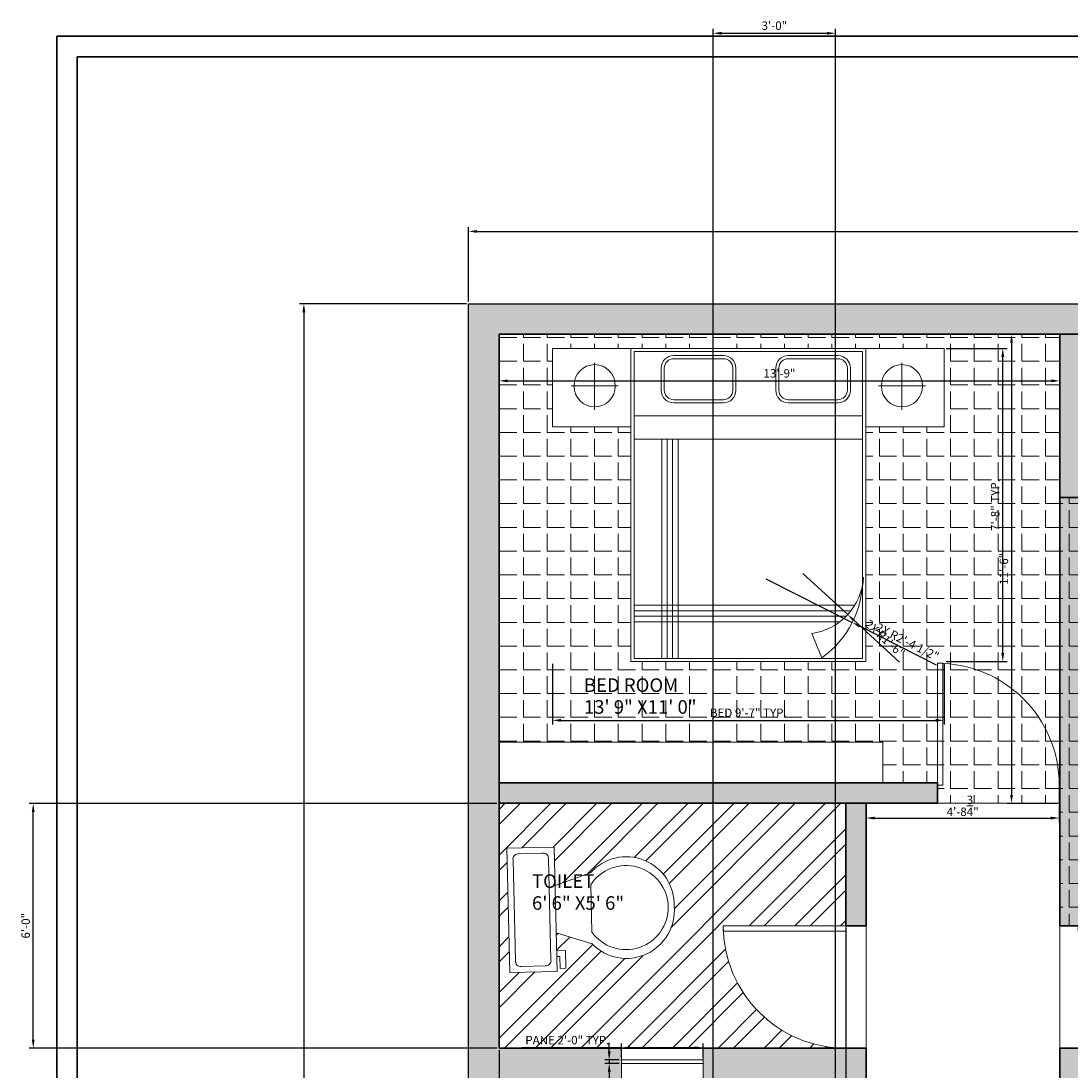
# Model space of a CAD drawing. Units: inches. Extents: x 2004 to 2661, y 1548 to 2351.
# Tile 4 of 5: x 2004 to 2312, y 2040 to 2349. Entities that reach past the tile are written whole.
import ezdxf

# ---------------------------------------------------------------- set-up
doc = ezdxf.new("R2010")
doc.units = ezdxf.units.IN
for name, color, linetype, lineweight in [('A-ANNO-DIMS', 2, 'Continuous', 18), ('A-ANNO-TTLB', 7, 'Continuous', 35), ('A-AREA-IDEN', 7, 'Continuous', 18), ('A-DOOR', 3, 'Continuous', 18), ('A-FLOR-CASE', 8, 'Continuous', 18), ('A-FLOR-FIXT', 9, 'Continuous', 18), ('A-FURN', 8, 'Continuous', 18), ('A-GLAZ', 4, 'Continuous', 18), ('A-WALL', 7, 'Continuous', 35), ('C-PROP', 7, 'Continuous', 25)]:
    doc.layers.add(name, color=color, linetype=linetype, lineweight=lineweight)
doc.layers.add('A-FLOR-PATT', color=18, linetype='Continuous', lineweight=13, true_color=0x000000)
doc.layers.add('A-WALL-PATT', color=18, linetype='Continuous', lineweight=13, true_color=0x000000)
doc.styles.get("Standard").update_dxf_attribs({"font": 'arial.ttf'})
doc.dimstyles.new('Copy of ISO-25', dxfattribs={"dimtxt": 2.5, "dimasz": 2.5, "dimexe": 1.25, "dimexo": 0.625, "dimtad": 1, "dimlunit": 4, "dimtxsty": 'Standard', "dimcen": 2.5, "dimadec": 0, "dimazin": 0, "dimtfac": 1, "dimtmove": 0, "dimatfit": 3, "dimfxl": 1, "dimarcsym": 0})

# ---------------------------------------------------------------- blocks, each defined once
blk = doc.blocks.new('*D1')
at = {"layer": 'A-ANNO-DIMS', "color": 0, "lineweight": -2, "transparency": 16777216}
for p, q in [((2135.26, 2266.72), (2135.26, 2288.6)), ((2137.76, 2287.35), (2528.76, 2287.35)), ((2531.26, 2266.72), (2531.26, 2288.6))]:
    blk.add_line(p, q, dxfattribs=at)
at = {"layer": 'A-ANNO-DIMS', "color": 0, "transparency": 16777216}
for points in [[(2137.76, 2287.77), (2137.76, 2286.93), (2135.26, 2287.35)], [(2528.76, 2287.77), (2528.76, 2286.93), (2531.26, 2287.35)]]:
    blk.add_solid(points, dxfattribs=at)
at = {"layer": 'Defpoints', "color": 0, "transparency": 16777216}
for p in [(2531.26, 2287.35), (2135.26, 2266.09), (2531.26, 2266.09)]:
    blk.add_point(p, dxfattribs=at)
at = {"layer": 'A-ANNO-DIMS', "color": 0, "transparency": 16777216, "insert": (2333.26, 2289.25), "char_height": 2.5, "attachment_point": 5}
blk.add_mtext("33'", dxfattribs=at)
blk = doc.blocks.new('A$C057D194F')
for p, q in [((0, 1.5, -0.1688), (0, 2, -0.1688)), ((0, 2, -0.1688), (0.5, 2, -0.1688)), ((0.5, 2, -0.1688), (0.5, 0, -0.1688)), ((2, 2, -0.1688), (0.5, 2, -0.1688)), ((1.98, 1.98, -0.1688), (0.52, 1.98, -0.1688)), ((0.52, 1.98, -0.1688), (0.52, 0.02, -0.1688)), ((1.0907, 1.9539, -0.1688), (0.7735, 1.9539, -0.1688)), ((1.8224, 1.9539, -0.1688), (1.5052, 1.9539, -0.1688)), ((1.98, 0.02, -0.1688), (1.98, 1.98, -0.1688)), ((2, 0, -0.1688), (2, 2, -0.1688)), ((2.5, 2, -0.1688), (2, 2, -0.1688)), ((2.5, 1.5, -0.1688), (2.5, 2, -0.1688)), ((0.2687, 1.9081, -0.1688), (0.2687, 1.761, -0.1688)), ((0.2687, 1.6081, -0.1688), (0.2687, 1.9081, -0.1688)), ((1.0907, 1.9339, -0.1688), (0.7735, 1.9339, -0.1688)), ((1.8224, 1.9339, -0.1688), (1.5052, 1.9339, -0.1688)), ((2.2313, 1.9081, -0.1688), (2.2313, 1.761, -0.1688)), ((2.2313, 1.6081, -0.1688), (2.2313, 1.9081, -0.1688)), ((0.6935, 1.8739, -0.1688), (0.6935, 1.7322, -0.1688)), ((0.7135, 1.8739, -0.1688), (0.7135, 1.7322, -0.1688)), ((1.1507, 1.7322, -0.1688), (1.1507, 1.8739, -0.1688)), ((1.1707, 1.7322, -0.1688), (1.1707, 1.8739, -0.1688)), ((1.4252, 1.8739, -0.1688), (1.4252, 1.7322, -0.1688)), ((1.4452, 1.8739, -0.1688), (1.4452, 1.7322, -0.1688)), ((1.8824, 1.7322, -0.1688), (1.8824, 1.8739, -0.1688)), ((1.9024, 1.7322, -0.1688), (1.9024, 1.8739, -0.1688)), ((0.4194, 1.761, -0.1688), (0.1194, 1.761, -0.1688)), ((0.2687, 1.761, -0.1688), (0.4194, 1.761, -0.1688)), ((0.2687, 1.761, -0.1688), (0.2687, 1.6081, -0.1688)), ((2.0806, 1.761, -0.1688), (2.3806, 1.761, -0.1688)), ((2.2313, 1.761, -0.1688), (2.0806, 1.761, -0.1688)), ((2.2313, 1.761, -0.1688), (2.2313, 1.6081, -0.1688)), ((0.7735, 1.6722, -0.1688), (1.0907, 1.6722, -0.1688)), ((0.7735, 1.6522, -0.1688), (1.0907, 1.6522, -0.1688)), ((1.5052, 1.6722, -0.1688), (1.8224, 1.6722, -0.1688)), ((1.5052, 1.6522, -0.1688), (1.8224, 1.6522, -0.1688)), ((1.98, 1.5693, -0.1688), (0.52, 1.5693, -0.1688)), ((0.5, 1.5, -0.1688), (0, 1.5, -0.1688)), ((2, 1.5, -0.1688), (2.5, 1.5, -0.1688)), ((1.98, 1.4193, -0.1688), (0.52, 1.4193, -0.1688)), ((0.6969, 0.02, -0.1688), (0.6969, 1.4193, -0.1688)), ((0.7319, 0.02, -0.1688), (0.7319, 1.4193, -0.1688)), ((0.7669, 0.02, -0.1688), (0.7669, 1.4193, -0.1688)), ((0.8019, 0.02, -0.1688), (0.8019, 1.4193, -0.1688)), ((0.52, 0.3595, -0.1688), (1.9292, 0.3595, -0.1688)), ((0.52, 0.3245, -0.1688), (1.905, 0.3245, -0.1688)), ((0.52, 0.2895, -0.1688), (1.8742, 0.2895, -0.1688)), ((0.52, 0.2545, -0.1688), (1.8344, 0.2545, -0.1688)), ((1.6548, 0.1789, -0.1688), (1.7198, 0.0251, -0.1688)), ((0.52, 0.02, -0.1688), (1.98, 0.02, -0.1688)), ((0.5, 0, -0.1688), (2, 0, -0.1688))]:
    blk.add_line(p, q)
for centre, radius, start, end in [((0.7735, 1.8739, -0.1688), 0.08, 90, 180), ((1.0907, 1.8739, -0.1688), 0.08, 0, 90), ((1.5052, 1.8739, -0.1688), 0.08, 90, 180), ((1.8224, 1.8739, -0.1688), 0.08, 0, 90), ((0.7735, 1.8739, -0.1688), 0.06, 90, 180), ((1.0907, 1.8739, -0.1688), 0.06, 0, 90), ((1.5052, 1.8739, -0.1688), 0.06, 90, 180), ((1.8224, 1.8739, -0.1688), 0.06, 0, 90), ((0.7735, 1.7322, -0.1688), 0.08, 180, 270), ((0.7735, 1.7322, -0.1688), 0.06, 180, 270), ((1.0907, 1.7322, -0.1688), 0.08, 270, 0), ((1.0907, 1.7322, -0.1688), 0.06, 270, 0), ((1.5052, 1.7322, -0.1688), 0.08, 180, 270), ((1.5052, 1.7322, -0.1688), 0.06, 180, 270), ((1.8224, 1.7322, -0.1688), 0.08, 270, 0), ((1.8224, 1.7322, -0.1688), 0.06, 270, 0), ((1.5992, 0.5623, -0.1688), 0.3874, 278.2518, 356.6808), ((1.363, 0.5286, -0.1688), 0.6171, 305.32946, 1.04595)]:
    blk.add_arc(centre, radius, start, end)
blk.add_ellipse((0.2687, 1.761, -0.1688), major_axis=(0, -0.1351), ratio=0.975448)
at = {"extrusion": (0, 0, -1)}
blk.add_ellipse((2.2313, 1.761, -0.1688), major_axis=(0, 0.1351), ratio=0.975448, dxfattribs=at)
for p in [(0.2687, 1.761, -0.1688), (2.2313, 1.761, -0.1688)]:
    blk.add_point(p)
blk = doc.blocks.new('*U5')
for p, q in [((0, 0), (0, -6)), ((40, 0), (40, -6))]:
    blk.add_line(p, q)
blk.add_lwpolyline([(0, 0), (0, 40), (1.75, 40), (1.75, 0)], close=True)
blk.add_arc((0, 0), 40, 0, 90)
blk = doc.blocks.new('*U8')
for p, q in [((0, 0), (0, -6)), ((-40, 0), (-40, -6))]:
    blk.add_line(p, q)
blk.add_lwpolyline([(0, 0), (0, 40), (-1.75, 40), (-1.75, 0)], close=True)
blk.add_arc((0, 0), 40, 90, 180)
blk = doc.blocks.new('*U7')
for p, q in [((-40, 0), (-40, 6)), ((0, 0), (0, 6))]:
    blk.add_line(p, q)
blk.add_lwpolyline([(0, 0), (0, -40), (-1.75, -40), (-1.75, 0)], close=True)
blk.add_arc((0, 0), 40, 180, 270)
blk = doc.blocks.new('*U10')
for p, q in [((241.3, -152.4), (241.3, -50.8)), ((-254, -215.9), (-203.2, -215.9)), ((-254, -241.3), (-254, -215.9)), ((-203.2, -215.9), (-203.2, -203.2)), ((-177.8, -203.2), (-177.8, -241.3)), ((-101.6, -203.2), (-152.4, -355.6)), ((101.6, -203.2), (152.4, -355.6)), ((-177.8, -241.3), (-254, -241.3)), ((101.6, -355.6), (-101.6, -355.6))]:
    blk.add_line(p, q)
blk.add_lwpolyline([(266.7, -203.2), (266.7, 0), (-266.7, 0), (-266.7, -203.2)], close=True)
for points in [[(215.9, -25.4), (-215.9, -25.4)], [(-241.3, -50.8), (-241.3, -152.4)], [(-215.9, -177.8), (215.9, -177.8)]]:
    blk.add_lwpolyline(points)
for centre, radius, start, end in [((-219.075, -47.625), 22.45064, 81.8699, 188.1301), ((219.075, -47.625), 22.45064, 351.8699, 98.1301), ((-219.075, -155.575), 22.45064, 171.869898, 278.1301), ((219.075, -155.575), 22.45064, 261.8699, 8.1301), ((-12.12088, -505.93752), 205.61935, 133.01722, 273.38), ((0.94996, -504.77674), 181.02486, 124.50543, 269.7), ((-0.94742, -504.77674), 181.02486, 270.3, 55.4946), ((12.12342, -505.93752), 205.61935, 266.62, 46.9828)]:
    blk.add_arc(centre, radius, start, end)
blk = doc.blocks.new('*D13')
at = {"layer": 'A-ANNO-DIMS', "color": 0, "lineweight": -2, "transparency": 16777216}
for p, q in [((2134.63, 2266.09), (2085.55, 2266.09)), ((2086.8, 2263.59), (2086.8, 1668.59)), ((2134.63, 1666.09), (2085.55, 1666.09))]:
    blk.add_line(p, q, dxfattribs=at)
at = {"layer": 'A-ANNO-DIMS', "color": 0, "transparency": 16777216}
for points in [[(2086.38, 2263.59), (2087.22, 2263.59), (2086.8, 2266.09)], [(2086.38, 1668.59), (2087.22, 1668.59), (2086.8, 1666.09)]]:
    blk.add_solid(points, dxfattribs=at)
at = {"layer": 'Defpoints', "color": 0, "transparency": 16777216}
for p in [(2135.26, 2266.09), (2086.8, 1666.09), (2135.26, 1666.09)]:
    blk.add_point(p, dxfattribs=at)
at = {"layer": 'A-ANNO-DIMS', "color": 0, "transparency": 16777216, "insert": (2084.9, 1966.09), "char_height": 2.5, "attachment_point": 5, "rotation": 90}
blk.add_mtext("50'", dxfattribs=at)
blk = doc.blocks.new('*D14')
at = {"layer": 'A-ANNO-DIMS', "color": 0, "lineweight": -2, "transparency": 16777216}
for p, q in [((2144.26, 2256.47), (2144.26, 2242.13)), ((2309.26, 2256.47), (2309.26, 2242.13)), ((2146.76, 2243.38), (2306.76, 2243.38))]:
    blk.add_line(p, q, dxfattribs=at)
at = {"layer": 'A-ANNO-DIMS', "color": 0, "transparency": 16777216}
for points in [[(2146.76, 2243.8), (2146.76, 2242.97), (2144.26, 2243.38)], [(2306.76, 2243.8), (2306.76, 2242.97), (2309.26, 2243.38)]]:
    blk.add_solid(points, dxfattribs=at)
at = {"layer": 'Defpoints', "color": 0, "transparency": 16777216}
for p in [(2144.26, 2257.09), (2309.26, 2257.09), (2309.26, 2243.38)]:
    blk.add_point(p, dxfattribs=at)
at = {"layer": 'A-ANNO-DIMS', "color": 0, "transparency": 16777216, "insert": (2226.76, 2245.28), "char_height": 2.5, "attachment_point": 5}
blk.add_mtext('13\'-9"', dxfattribs=at)
blk = doc.blocks.new('*D15')
at = {"layer": 'A-ANNO-DIMS', "color": 0, "lineweight": -2, "transparency": 16777216}
for p, q in [((2308.63, 2257.09), (2293.79, 2257.09)), ((2295.04, 2254.59), (2295.04, 2121.59)), ((2308.63, 2119.09), (2293.79, 2119.09))]:
    blk.add_line(p, q, dxfattribs=at)
at = {"layer": 'A-ANNO-DIMS', "color": 0, "transparency": 16777216}
for points in [[(2294.62, 2254.59), (2295.45, 2254.59), (2295.04, 2257.09)], [(2294.62, 2121.59), (2295.45, 2121.59), (2295.04, 2119.09)]]:
    blk.add_solid(points, dxfattribs=at)
at = {"layer": 'Defpoints', "color": 0, "transparency": 16777216}
for p in [(2309.26, 2257.09), (2295.04, 2119.09), (2309.26, 2119.09)]:
    blk.add_point(p, dxfattribs=at)
at = {"layer": 'A-ANNO-DIMS', "color": 0, "transparency": 16777216, "insert": (2293.13, 2188.09), "char_height": 2.5, "attachment_point": 5, "rotation": 90}
blk.add_mtext('11\'-6"', dxfattribs=at)
blk = doc.blocks.new('*D16')
at = {"layer": 'A-ANNO-DIMS', "color": 0, "lineweight": -2, "transparency": 16777216}
for p, q in [((2252.26, 2118.47), (2252.26, 2113.51)), ((2309.08, 2118.47), (2309.08, 2113.51)), ((2254.76, 2114.76), (2306.58, 2114.76))]:
    blk.add_line(p, q, dxfattribs=at)
at = {"layer": 'A-ANNO-DIMS', "color": 0, "transparency": 16777216}
for points in [[(2254.76, 2115.18), (2254.76, 2114.34), (2252.26, 2114.76)], [(2306.58, 2115.18), (2306.58, 2114.34), (2309.08, 2114.76)]]:
    blk.add_solid(points, dxfattribs=at)
at = {"layer": 'Defpoints', "color": 0, "transparency": 16777216}
for p in [(2252.26, 2119.09), (2309.08, 2119.09), (2309.08, 2114.76)]:
    blk.add_point(p, dxfattribs=at)
at = {"layer": 'A-ANNO-DIMS', "color": 0, "transparency": 16777216, "insert": (2280.67, 2118.35), "char_height": 2.5, "attachment_point": 5}
blk.add_mtext('4\'-8{\\H1x;\\S3/4;}"', dxfattribs=at)
blk = doc.blocks.new('WINDOW-PANE-24IN')
for p, q in [((0, 1), (24, 1)), ((0, 0), (24, 0))]:
    blk.add_line(p, q)
blk = doc.blocks.new('*D29')
at = {"layer": 'A-ANNO-DIMS', "color": 0, "lineweight": -2, "transparency": 16777216}
for p, q in [((2159.99, 2160.16), (2159.99, 2142.26)), ((2275.19, 2160.16), (2275.19, 2142.26)), ((2162.49, 2143.51), (2272.69, 2143.51))]:
    blk.add_line(p, q, dxfattribs=at)
at = {"layer": 'A-ANNO-DIMS', "color": 0, "transparency": 16777216}
for points in [[(2162.49, 2143.92), (2162.49, 2143.09), (2159.99, 2143.51)], [(2272.69, 2143.92), (2272.69, 2143.09), (2275.19, 2143.51)]]:
    blk.add_solid(points, dxfattribs=at)
at = {"layer": 'Defpoints', "color": 0, "transparency": 16777216}
for p in [(2159.99, 2160.79), (2275.19, 2160.79), (2275.19, 2143.51)]:
    blk.add_point(p, dxfattribs=at)
at = {"layer": 'A-ANNO-DIMS', "color": 0, "transparency": 16777216, "insert": (2217.59, 2145.41), "char_height": 2.5, "attachment_point": 5}
blk.add_mtext('BED 9\'-7" TYP.', dxfattribs=at)
blk = doc.blocks.new('*D30')
at = {"layer": 'A-ANNO-DIMS', "color": 0, "lineweight": -2, "transparency": 16777216}
for p, q in [((2275.81, 2252.95), (2293.72, 2252.95)), ((2292.47, 2163.29), (2292.47, 2250.45)), ((2275.81, 2160.79), (2293.72, 2160.79))]:
    blk.add_line(p, q, dxfattribs=at)
at = {"layer": 'A-ANNO-DIMS', "color": 0, "transparency": 16777216}
for points in [[(2292.05, 2250.45), (2292.89, 2250.45), (2292.47, 2252.95)], [(2292.05, 2163.29), (2292.89, 2163.29), (2292.47, 2160.79)]]:
    blk.add_solid(points, dxfattribs=at)
at = {"layer": 'Defpoints', "color": 0, "transparency": 16777216}
for p in [(2275.19, 2252.95), (2292.47, 2252.95), (2275.19, 2160.79)]:
    blk.add_point(p, dxfattribs=at)
at = {"layer": 'A-ANNO-DIMS', "color": 0, "transparency": 16777216, "insert": (2290.57, 2206.87), "char_height": 2.5, "attachment_point": 5, "rotation": 90}
blk.add_mtext('7\'-8" TYP.', dxfattribs=at)
blk = doc.blocks.new('*D35')
at = {"layer": 'A-ANNO-DIMS', "color": 0, "lineweight": -2, "transparency": 16777216}
for p, q in [((2180.26, 2044.22), (2180.26, 2048.44)), ((2204.26, 2044.22), (2204.26, 2048.44)), ((2180.26, 2047.19), (2150.91, 2047.19)), ((2201.76, 2047.19), (2182.76, 2047.19))]:
    blk.add_line(p, q, dxfattribs=at)
at = {"layer": 'A-ANNO-DIMS', "color": 0, "transparency": 16777216}
for points in [[(2182.76, 2047.61), (2182.76, 2046.78), (2180.26, 2047.19)], [(2201.76, 2047.61), (2201.76, 2046.78), (2204.26, 2047.19)]]:
    blk.add_solid(points, dxfattribs=at)
at = {"layer": 'Defpoints', "color": 0, "transparency": 16777216}
for p in [(2180.26, 2047.19), (2180.26, 2043.59), (2204.26, 2043.59)]:
    blk.add_point(p, dxfattribs=at)
at = {"layer": 'A-ANNO-DIMS', "color": 0, "transparency": 16777216, "insert": (2164.33, 2049.09), "char_height": 2.5, "attachment_point": 5}
blk.add_mtext('PANE 2\'-0" TYP.', dxfattribs=at)
blk = doc.blocks.new('*D36')
at = {"layer": 'A-ANNO-DIMS', "color": 0, "lineweight": -2, "transparency": 16777216}
for p, q in [((2176.66, 2046.09), (2176.66, 2048.59)), ((2179.63, 2043.59), (2175.41, 2043.59)), ((2179.63, 2042.59), (2175.41, 2042.59)), ((2176.66, 2043.59), (2176.66, 2042.59)), ((2176.66, 2040.09), (2176.66, 2021.1))]:
    blk.add_line(p, q, dxfattribs=at)
at = {"layer": 'A-ANNO-DIMS', "color": 0, "transparency": 16777216}
for points in [[(2176.24, 2046.09), (2177.07, 2046.09), (2176.66, 2043.59)], [(2176.24, 2040.09), (2177.07, 2040.09), (2176.66, 2042.59)]]:
    blk.add_solid(points, dxfattribs=at)
at = {"layer": 'Defpoints', "color": 0, "transparency": 16777216}
for p in [(2176.66, 2042.59), (2180.26, 2043.59), (2180.26, 2042.59)]:
    blk.add_point(p, dxfattribs=at)
at = {"layer": 'A-ANNO-DIMS', "color": 0, "transparency": 16777216, "insert": (2174.76, 2029.35), "char_height": 2.5, "attachment_point": 5, "rotation": 90}
blk.add_mtext('0\'-1" TYP.', dxfattribs=at)
blk = doc.blocks.new('*D37')
at = {"layer": 'A-ANNO-DIMS', "color": 0, "lineweight": -2, "transparency": 16777216}
for p, q in [((2246.26, 2082.47), (2246.26, 1630.09)), ((2144.26, 2046.47), (2144.26, 1630.09)), ((2146.76, 1631.34), (2243.76, 1631.34))]:
    blk.add_line(p, q, dxfattribs=at)
at = {"layer": 'A-ANNO-DIMS', "color": 0, "transparency": 16777216}
for points in [[(2146.76, 1631.76), (2146.76, 1630.93), (2144.26, 1631.34)], [(2243.76, 1631.76), (2243.76, 1630.93), (2246.26, 1631.34)]]:
    blk.add_solid(points, dxfattribs=at)
at = {"layer": 'Defpoints', "color": 0, "transparency": 16777216}
for p in [(2246.26, 2083.09), (2144.26, 2047.09), (2246.26, 1631.34)]:
    blk.add_point(p, dxfattribs=at)
at = {"layer": 'A-ANNO-DIMS', "color": 0, "transparency": 16777216, "insert": (2195.26, 1633.24), "char_height": 2.5, "attachment_point": 5}
blk.add_mtext('8\'-6"', dxfattribs=at)
blk = doc.blocks.new('*D38')
at = {"layer": 'A-ANNO-DIMS', "color": 0, "lineweight": -2, "transparency": 16777216}
for p, q in [((2143.63, 2119.09), (2005.91, 2119.09)), ((2007.16, 2049.59), (2007.16, 2116.59)), ((2143.63, 2047.09), (2005.91, 2047.09))]:
    blk.add_line(p, q, dxfattribs=at)
at = {"layer": 'A-ANNO-DIMS', "color": 0, "transparency": 16777216}
for points in [[(2006.74, 2116.59), (2007.57, 2116.59), (2007.16, 2119.09)], [(2006.74, 2049.59), (2007.57, 2049.59), (2007.16, 2047.09)]]:
    blk.add_solid(points, dxfattribs=at)
at = {"layer": 'Defpoints', "color": 0, "transparency": 16777216}
for p in [(2007.16, 2119.09), (2144.26, 2119.09), (2144.26, 2047.09)]:
    blk.add_point(p, dxfattribs=at)
at = {"layer": 'A-ANNO-DIMS', "color": 0, "transparency": 16777216, "insert": (2005.26, 2083.09), "char_height": 2.5, "attachment_point": 5, "rotation": 90}
blk.add_mtext('6\'-0"', dxfattribs=at)
blk = doc.blocks.new('*D46')
at = {"layer": 'A-ANNO-DIMS', "color": 0, "lineweight": -2, "transparency": 16777216}
for p, q in [((2207.26, 1879.72), (2207.26, 2346.91)), ((2209.76, 2345.66), (2240.76, 2345.66)), ((2243.26, 1879.72), (2243.26, 2346.91))]:
    blk.add_line(p, q, dxfattribs=at)
at = {"layer": 'A-ANNO-DIMS', "color": 0, "transparency": 16777216}
for points in [[(2209.76, 2346.07), (2209.76, 2345.24), (2207.26, 2345.66)], [(2240.76, 2346.07), (2240.76, 2345.24), (2243.26, 2345.66)]]:
    blk.add_solid(points, dxfattribs=at)
at = {"layer": 'Defpoints', "color": 0, "transparency": 16777216}
for p in [(2243.26, 2345.66), (2207.26, 1879.09), (2243.26, 1879.09)]:
    blk.add_point(p, dxfattribs=at)
at = {"layer": 'A-ANNO-DIMS', "color": 0, "transparency": 16777216, "insert": (2225.26, 2347.56), "char_height": 2.5, "attachment_point": 5}
blk.add_mtext('3\'-0"', dxfattribs=at)
blk = doc.blocks.new('*D54')
at = {"layer": 'A-ANNO-DIMS', "color": 0, "lineweight": -2, "transparency": 16777216}
for p, q in [((2222.79, 2185.14), (2248.18, 2172.32)), ((2273.01, 2159.77), (2250.41, 2171.19))]:
    blk.add_line(p, q, dxfattribs=at)
at = {"layer": 'A-ANNO-DIMS', "color": 0, "transparency": 16777216}
blk.add_solid([(2250.59, 2171.56), (2250.22, 2170.82), (2248.18, 2172.32)], dxfattribs=at)
at = {"layer": 'Defpoints', "color": 0, "transparency": 16777216}
for p in [(2222.79, 2185.14), (2248.18, 2172.32)]:
    blk.add_point(p, dxfattribs=at)
at = {"layer": 'A-ANNO-DIMS', "color": 0, "transparency": 16777216, "insert": (2264.27, 2166.33), "char_height": 2.5, "attachment_point": 5, "rotation": 333.1884}
blk.add_mtext('2X R2\'-4 1/2"', dxfattribs=at)
blk = doc.blocks.new('*D55')
at = {"layer": 'A-ANNO-DIMS', "color": 0, "lineweight": -2, "transparency": 16777216}
for p, q in [((2233.68, 2186.7), (2246.83, 2174.63)), ((2262.09, 2160.63), (2248.68, 2172.94))]:
    blk.add_line(p, q, dxfattribs=at)
at = {"layer": 'A-ANNO-DIMS', "color": 0, "transparency": 16777216}
blk.add_solid([(2248.96, 2173.25), (2248.39, 2172.63), (2246.83, 2174.63)], dxfattribs=at)
at = {"layer": 'Defpoints', "color": 0, "transparency": 16777216}
for p in [(2233.68, 2186.7), (2246.83, 2174.63)]:
    blk.add_point(p, dxfattribs=at)
at = {"layer": 'A-ANNO-DIMS', "color": 0, "transparency": 16777216, "insert": (2257.59, 2167.34), "char_height": 2.5, "attachment_point": 5, "rotation": 317.4671}
blk.add_mtext('2X R1\'-6"', dxfattribs=at)

msp = doc.modelspace()

# ---------------------------------------------------------------- hatches: boundary and pattern name
at = {"layer": 'A-FLOR-PATT'}
h = msp.add_hatch(dxfattribs=at)
h.set_pattern_fill('ANSI32', color=256)
h.paths.add_polyline_path([(2522.257, 2257.093), (2466.833, 2257.093), (2315.257, 2257.093), (2418.757, 2233.093)])
h.paths.add_polyline_path([(2418.757, 2233.093), (2315.257, 2257.093), (2315.257, 2209.093)])
h.paths.add_polyline_path([(2418.757, 2233.093), (2315.257, 2209.093), (2522.257, 2209.093)])
h.paths.add_polyline_path([(2522.257, 2257.093), (2418.757, 2233.093), (2522.257, 2209.093)])
h.paths.add_polyline_path([(2522.257, 1753.093), (2318.257, 1753.093), (2318.257, 1675.093), (2522.257, 1675.093)])
h.paths.add_polyline_path([(2210.267, 2081.517), (2210.233, 2081.517), (2210.233, 2083.093), (2246.257, 2083.093), (2246.257, 2119.093), (2144.257, 2119.093), (2144.257, 2047.093), (2244.938, 2047.093, -0.390864)])
h.paths.add_polyline_path([(2171.613, 2077.721), (2161.069, 2080.96), (2161.193, 2075.729), (2163.808, 2075.791), (2163.932, 2070.56), (2162.189, 2070.519), (2162.106, 2074.006), (2161.234, 2073.986), (2161.338, 2069.627), (2147.389, 2069.296), (2146.521, 2105.911), (2160.469, 2106.241), (2160.738, 2094.908), (2171.117, 2098.643, -0.7025712), (2195.775, 2088.761, -0.7025621)], flags=16)
h.paths.add_polyline_path([(2171.53, 2081.208), (2171.2, 2095.156, -0.7345333), (2194.031, 2088.72, -0.7345297)], flags=0)
h.paths.add_polyline_path([(2158.245, 2071.298), (2150.835, 2071.122, -0.4142136), (2149.061, 2072.388), (2148.347, 2102.465, -0.4142136), (2149.614, 2104.239), (2157.024, 2104.415, -0.4142136), (2158.798, 2103.149), (2159.512, 2073.072, -0.4142136)], flags=0)
h.paths.add_polyline_path([(2522.257, 2200.093), (2517.397, 2200.093), (2517.397, 2185.232), (2505.384, 2185.232), (2509.08, 2174.143, -0.7025712), (2497.991, 2148.268, -0.7025621), (2486.902, 2174.142), (2490.599, 2185.232), (2485.054, 2185.232), (2485.054, 2182.459), (2479.509, 2182.459), (2479.509, 2184.307), (2483.206, 2184.307), (2483.206, 2185.232), (2478.585, 2185.232), (2478.585, 2200.093), (2459.257, 2200.093), (2459.257, 2106.686, -0.3761573), (2493.676, 2139.619), (2493.676, 2139.653), (2495.257, 2139.653), (2495.257, 2104.093), (2522.257, 2104.093)])
h.paths.add_polyline_path([(2349.854, 1719.146), (2381.921, 1719.146), (2381.921, 1725.273), (2349.854, 1725.273)], flags=24)
h.paths.add_polyline_path([(2349.84, 1725.558), (2388.851, 1725.558), (2388.851, 1731.767), (2349.84, 1731.767)], flags=24)
h.paths.add_polyline_path([(2152.908, 2086.679), (2181.867, 2086.679), (2181.867, 2092.806), (2152.908, 2092.806)], flags=8)
h.paths.add_polyline_path([(2152.895, 2093.091), (2174.525, 2093.091), (2174.525, 2099.3), (2152.895, 2099.3)], flags=8)
h.paths.add_polyline_path([(2515.001, 2150.174), (2515.001, 2154.033), (2509.85, 2154.033), (2509.85, 2150.174)], flags=24)
h.paths.add_polyline_path([(2469.272, 2171.563), (2498.231, 2171.563), (2498.231, 2177.69), (2469.272, 2177.69)], flags=24)
h.paths.add_polyline_path([(2469.258, 2177.975), (2490.888, 2177.975), (2490.888, 2184.184), (2469.258, 2184.184)], flags=24)
h = msp.add_hatch(dxfattribs=at)
h.set_pattern_fill('ANGLE', color=256)
h.set_pattern_definition([(0, (0, 0), (0, 6.985), [5.08, -1.905]), (90, (0, 0), (-6.985, 4e-16), [5.08, -1.905])])
h.paths.add_polyline_path([(2453.257, 2092.093), (2453.257, 2200.093), (2368.773, 2200.093), (2368.773, 2209.093), (2315.257, 2209.093), (2309.257, 2209.093), (2309.257, 2119.093), (2309.257, 2083.093), (2315.257, 2083.093), (2350.837, 2083.093), (2350.837, 2081.511), (2350.802, 2081.511, -0.3968312), (2315.257, 2046.941), (2315.257, 2044.093), (2453.257, 2044.093), (2453.257, 2056.093)])
h.paths.add_polyline_path([(2338.94, 2106.763), (2338.94, 2083.722), (2315.9, 2083.722), (2315.9, 2106.763), (2315.9, 2175.884), (2315.9, 2198.924), (2338.94, 2198.924), (2338.94, 2175.884), (2408.062, 2175.884), (2408.062, 2106.763)], flags=16)
h.paths.add_polyline_path([(2316.822, 2107.684), (2316.822, 2174.962), (2383.185, 2174.962, -0.0091279), (2384.223, 2174.962), (2407.14, 2174.962), (2407.14, 2107.684)], flags=0)
h.paths.add_polyline_path([(2342.657, 2115.838), (2342.657, 2120.677), (2391.497, 2120.677), (2391.497, 2172.623, -0.0921038), (2396.336, 2168.251), (2396.336, 2115.838)], flags=0)
h.paths.add_polyline_path([(2393.11, 2119.064), (2394.723, 2119.064), (2394.723, 2117.451), (2393.11, 2117.451)], flags=0)
edge = h.paths.add_edge_path(flags=0)
edge.add_ellipse((2326.912, 2096.106), major_axis=(-6.224, 0), ratio=0.9754478, start_angle=450, end_angle=540, ccw=False)
edge.add_ellipse((2326.912, 2096.106), major_axis=(-6.224, 0), ratio=0.9754478, start_angle=360, end_angle=450, ccw=False)
edge.add_ellipse((2326.912, 2096.106), major_axis=(-6.224, 0), ratio=0.9754478, start_angle=270, end_angle=360, ccw=False)
edge.add_ellipse((2326.912, 2096.106), major_axis=(-6.224, 0), ratio=0.9754478, start_angle=180, end_angle=270, ccw=False)
h.paths.add_polyline_path([(2328.241, 2115.678), (2321.709, 2115.678, -0.4142136), (2318.023, 2119.364), (2318.023, 2133.984, -0.4142136), (2321.709, 2137.671), (2328.241, 2137.671, -0.4142136), (2331.928, 2133.984), (2331.928, 2119.364, -0.4142136)], flags=0)
h.paths.add_polyline_path([(2328.241, 2116.599), (2321.709, 2116.599, -0.4142136), (2318.945, 2119.364), (2318.945, 2133.984, -0.4142136), (2321.709, 2136.749), (2328.241, 2136.749, -0.4142136), (2331.006, 2133.984), (2331.006, 2119.364, -0.4142136)], flags=0)
h.paths.add_polyline_path([(2328.241, 2149.395), (2321.709, 2149.395, -0.4142136), (2318.023, 2153.081), (2318.023, 2167.701, -0.4142136), (2321.709, 2171.388), (2328.241, 2171.388, -0.4142136), (2331.928, 2167.701), (2331.928, 2153.081, -0.4142136)], flags=0)
h.paths.add_polyline_path([(2328.241, 2150.316), (2321.709, 2150.316, -0.4142136), (2318.945, 2153.081), (2318.945, 2167.701, -0.4142136), (2321.709, 2170.466), (2328.241, 2170.466, -0.4142136), (2331.006, 2167.701), (2331.006, 2153.081, -0.4142136)], flags=0)
edge = h.paths.add_edge_path(flags=0)
edge.add_ellipse((2326.912, 2186.54), major_axis=(-6.224, 0), ratio=0.9754478, start_angle=0, end_angle=90, ccw=False)
edge.add_ellipse((2326.912, 2186.54), major_axis=(-6.224, 0), ratio=0.9754478, start_angle=270, end_angle=360, ccw=False)
edge.add_ellipse((2326.912, 2186.54), major_axis=(-6.224, 0), ratio=0.9754478, start_angle=180, end_angle=270, ccw=False)
edge.add_ellipse((2326.912, 2186.54), major_axis=(-6.224, 0), ratio=0.9754478, start_angle=90, end_angle=180, ccw=False)
h.paths.add_polyline_path([(2309.257, 2209.093), (2309.257, 2257.093), (2144.257, 2257.093), (2144.257, 2137.093), (2257.19, 2137.093), (2257.19, 2125.093), (2273.257, 2125.093), (2273.257, 2119.093), (2309.257, 2119.093)])
h.paths.add_polyline_path([(2183.028, 2229.908), (2159.988, 2229.908), (2159.988, 2252.949), (2183.028, 2252.949), (2252.149, 2252.949), (2275.19, 2252.949), (2275.19, 2229.908), (2252.149, 2229.908), (2252.149, 2160.787), (2183.028, 2160.787)], flags=16)
h.paths.add_polyline_path([(2183.95, 2252.027), (2251.228, 2252.027), (2251.228, 2185.663, -0.0091279), (2251.228, 2184.625), (2251.228, 2161.709), (2183.95, 2161.709)], flags=0)
h.paths.add_polyline_path([(2192.104, 2172.513), (2192.104, 2226.192), (2196.942, 2226.192), (2196.942, 2177.351), (2248.888, 2177.351, -0.0921038), (2244.517, 2172.513)], flags=0)
h.paths.add_polyline_path([(2193.716, 2174.125), (2193.716, 2175.738), (2195.329, 2175.738), (2195.329, 2174.125)], flags=0)
edge = h.paths.add_edge_path(flags=0)
edge.add_ellipse((2172.372, 2241.936), major_axis=(0, 6.224), ratio=0.9754478, start_angle=450, end_angle=540, ccw=False)
edge.add_ellipse((2172.372, 2241.936), major_axis=(0, 6.224), ratio=0.9754478, start_angle=360, end_angle=450, ccw=False)
edge.add_ellipse((2172.372, 2241.936), major_axis=(0, 6.224), ratio=0.9754478, start_angle=270, end_angle=360, ccw=False)
edge.add_ellipse((2172.372, 2241.936), major_axis=(0, 6.224), ratio=0.9754478, start_angle=180, end_angle=270, ccw=False)
h.paths.add_polyline_path([(2191.943, 2240.607), (2191.943, 2247.139, -0.4142136), (2195.63, 2250.826), (2210.25, 2250.826, -0.4142136), (2213.936, 2247.139), (2213.936, 2240.607, -0.4142136), (2210.25, 2236.921), (2195.63, 2236.921, -0.4142136)], flags=0)
h.paths.add_polyline_path([(2192.865, 2240.607), (2192.865, 2247.139, -0.4142136), (2195.63, 2249.904), (2210.25, 2249.904, -0.4142136), (2213.015, 2247.139), (2213.015, 2240.607, -0.4142136), (2210.25, 2237.842), (2195.63, 2237.842, -0.4142136)], flags=0)
h.paths.add_polyline_path([(2225.66, 2240.607), (2225.66, 2247.139, -0.4142136), (2229.347, 2250.826), (2243.967, 2250.826, -0.4142136), (2247.653, 2247.139), (2247.653, 2240.607, -0.4142136), (2243.967, 2236.921), (2229.347, 2236.921, -0.4142136)], flags=0)
h.paths.add_polyline_path([(2226.582, 2240.607), (2226.582, 2247.139, -0.4142136), (2229.347, 2249.904), (2243.967, 2249.904, -0.4142136), (2246.732, 2247.139), (2246.732, 2240.607, -0.4142136), (2243.967, 2237.842), (2229.347, 2237.842, -0.4142136)], flags=0)
edge = h.paths.add_edge_path(flags=0)
edge.add_ellipse((2262.806, 2241.936), major_axis=(0, 6.224), ratio=0.9754478, start_angle=90, end_angle=180, ccw=False)
edge.add_ellipse((2262.806, 2241.936), major_axis=(0, 6.224), ratio=0.9754478, start_angle=0, end_angle=90, ccw=False)
edge.add_ellipse((2262.806, 2241.936), major_axis=(0, 6.224), ratio=0.9754478, start_angle=270, end_angle=360, ccw=False)
edge.add_ellipse((2262.806, 2241.936), major_axis=(0, 6.224), ratio=0.9754478, start_angle=180, end_angle=270, ccw=False)
at = {"layer": 'A-WALL-PATT'}
h = msp.add_hatch(color=256, dxfattribs=at)
h.dxf.hatch_style = 1
h.paths.add_polyline_path([(2315.257, 2266.093), (2135.257, 2266.093), (2135.257, 1666.093), (2531.257, 1666.093), (2531.257, 1753.093), (2522.257, 1753.093), (2522.257, 1675.093), (2144.257, 1675.093), (2144.257, 2038.093), (2180.257, 2038.093), (2180.257, 2047.093), (2144.257, 2047.093), (2144.257, 2257.093), (2309.257, 2257.093), (2315.257, 2257.093)])
h.paths.add_polyline_path([(2522.257, 2266.093), (2315.257, 2266.093), (2315.257, 2257.093), (2522.257, 2257.093)], flags=17)
h.paths.add_polyline_path([(2368.773, 2209.093), (2315.257, 2209.093), (2309.257, 2209.093), (2309.257, 2119.093), (2309.257, 2083.093), (2315.257, 2083.093), (2315.257, 2119.093), (2315.257, 2200.093), (2368.773, 2200.093)], flags=17)
h.paths.add_polyline_path([(2459.257, 2209.093), (2428.773, 2209.093), (2428.773, 2200.093), (2453.257, 2200.093), (2459.257, 2200.093)], flags=17)
h.paths.add_polyline_path([(2522.257, 2209.093), (2483.257, 2209.093), (2483.257, 2200.093), (2522.257, 2200.093)], flags=17)
h.paths.add_polyline_path([(2522.257, 2044.093), (2459.257, 2044.093), (2459.257, 2056.073, -0.004139), (2458.66, 2056.069), (2453.257, 2056.069), (2453.257, 2044.093), (2315.257, 2044.093), (2315.257, 2046.941, -0.0039864), (2314.68, 2046.936), (2309.257, 2046.936), (2309.257, 2038.093), (2315.257, 2038.093), (2522.257, 2038.093)], flags=17)
h.paths.add_polyline_path([(2531.257, 2266.093), (2522.257, 2266.093), (2522.257, 2257.093), (2522.257, 2209.093), (2522.257, 2200.093), (2522.257, 2104.093), (2522.257, 1762.093), (2498.257, 1762.093), (2498.257, 1753.093), (2522.257, 1753.093), (2531.257, 1753.093)], flags=17)
h.paths.add_polyline_path([(2522.257, 2104.093), (2495.257, 2104.093), (2495.257, 2103.514), (2495.257, 2098.093), (2503.401, 2098.093), (2522.257, 2098.093)], flags=17)
h.paths.add_polyline_path([(2455.748, 2073.874), (2484.708, 2073.874), (2484.708, 2080.001), (2455.748, 2080.001)], flags=25)
h.paths.add_polyline_path([(2455.735, 2080.287), (2477.056, 2080.287), (2477.056, 2086.492), (2455.735, 2086.492)], flags=25)
h.paths.add_polyline_path([(2469.272, 2171.563), (2498.231, 2171.563), (2498.231, 2177.69), (2469.272, 2177.69)], flags=25)
h.paths.add_polyline_path([(2469.258, 2177.975), (2490.888, 2177.975), (2490.888, 2184.184), (2469.258, 2184.184)], flags=25)
h.paths.add_polyline_path([(2360.849, 2078.511), (2396.023, 2078.511), (2396.023, 2084.638), (2360.849, 2084.638)], flags=25)
h.paths.add_polyline_path([(2360.835, 2084.923), (2394.883, 2084.923), (2394.883, 2091.132), (2360.835, 2091.132)], flags=25)
h = msp.add_hatch(color=256, dxfattribs=at)
h.dxf.hatch_style = 1
h.paths.add_polyline_path([(2252.257, 2038.093), (2252.257, 2047.093), (2246.257, 2047.093), (2204.257, 2047.093), (2204.257, 2038.093), (2243.257, 2038.093), (2243.257, 1888.093), (2243.257, 1879.093), (2273.257, 1879.093), (2273.257, 1888.093), (2252.257, 1888.093)])
h.paths.add_polyline_path([(2273.257, 2125.093), (2144.257, 2125.093), (2144.257, 2119.093), (2246.257, 2119.093), (2273.257, 2119.093)])
h.paths.add_polyline_path([(2459.257, 2200.093), (2453.257, 2200.093), (2453.257, 2092.093), (2459.257, 2092.093)])
h.paths.add_polyline_path([(2522.257, 1888.093), (2426.257, 1888.093), (2426.257, 1882.093), (2522.257, 1882.093)])
h.paths.add_polyline_path([(2460.257, 1834.093), (2454.257, 1834.093), (2454.257, 1762.093), (2460.257, 1762.093)])
h.paths.add_polyline_path([(2460.257, 1882.093), (2454.257, 1882.093), (2454.257, 1870.093), (2460.257, 1870.093)])
h.paths.add_polyline_path([(2462.257, 1762.093), (2460.257, 1762.093), (2454.257, 1762.093), (2390.257, 1762.093), (2390.257, 1753.093), (2462.257, 1753.093)])
h.paths.add_polyline_path([(2342.257, 1762.093), (2318.257, 1762.093), (2318.257, 1882.093), (2318.257, 1888.093), (2309.257, 1888.093), (2309.257, 1879.093), (2309.257, 1753.093), (2318.257, 1753.093), (2342.257, 1753.093)])
h.paths.add_polyline_path([(2354.257, 1888.093), (2318.257, 1888.093), (2318.257, 1882.093), (2354.257, 1882.093)])
h.paths.add_polyline_path([(2318.257, 1753.093), (2309.257, 1753.093), (2309.257, 1675.093), (2318.257, 1675.093)])
h.paths.add_polyline_path([(2207.257, 1884.43), (2207.257, 1888.093), (2183.257, 1888.093), (2183.257, 1879.093), (2207.257, 1879.093)])
h.paths.add_polyline_path([(2252.257, 2119.093), (2246.257, 2119.093), (2246.257, 2083.093), (2251.66, 2083.093), (2252.257, 2083.093)])
h.paths.add_polyline_path([(2315.257, 2257.093), (2309.257, 2257.093), (2309.257, 2209.093), (2315.257, 2209.093)])

# ---------------------------------------------------------------- linework, layer by layer
at = {"layer": 'A-ANNO-TTLB'}
for points in [[(2014.058, 2344.754), (2661.447, 2344.754), (2661.447, 1548.19), (2014.058, 1548.19)], [(2020.058, 2338.754), (2655.447, 2338.754), (2655.447, 1554.19), (2020.058, 1554.19)]]:
    msp.add_lwpolyline(points, close=True, dxfattribs=at)
at = {"layer": 'A-DOOR'}
for p, q in [((2273.257, 2119.093), (2309.257, 2119.093)), ((2252.257, 2083.093), (2252.257, 2047.093)), ((2309.257, 2083.093), (2309.257, 2047.093))]:
    msp.add_line(p, q, dxfattribs=at)
at = {"layer": 'A-FLOR-CASE'}
for p, q in [((2144.257, 2125.093), (2144.257, 2137.093)), ((2144.257, 2137.093), (2257.19, 2137.093)), ((2257.19, 2137.093), (2257.19, 2125.093))]:
    msp.add_line(p, q, dxfattribs=at)
at = {"layer": 'A-GLAZ'}
for p, q in [((2180.257, 2038.093), (2180.257, 2047.093)), ((2204.257, 2038.093), (2204.257, 2047.093))]:
    msp.add_line(p, q, dxfattribs=at)
at = {"layer": 'A-WALL'}
for p, q in [((2144.257, 2257.093), (2309.257, 2257.093)), ((2144.257, 2257.093), (2309.257, 2257.093)), ((2144.257, 2257.093), (2144.257, 2125.093)), ((2144.257, 2047.093), (2144.257, 2257.093)), ((2309.257, 2119.093), (2309.257, 2257.093)), ((2309.257, 2257.093), (2315.257, 2257.093)), ((2315.257, 2209.093), (2309.257, 2209.093)), ((2144.257, 2125.093), (2273.257, 2125.093)), ((2273.257, 2119.093), (2273.257, 2125.093)), ((2273.257, 2119.093), (2144.257, 2119.093)), ((2144.257, 2119.093), (2246.257, 2119.093)), ((2246.257, 2119.093), (2246.257, 2083.093)), ((2252.257, 2083.093), (2252.257, 2119.093)), ((2309.257, 2083.093), (2309.257, 2119.093)), ((2252.257, 2083.093), (2246.257, 2083.093)), ((2246.257, 2083.093), (2246.257, 2083.093)), ((2309.257, 2083.093), (2315.257, 2083.093)), ((2246.257, 2047.093), (2144.257, 2047.093)), ((2246.257, 2047.093), (2252.257, 2047.093)), ((2252.257, 2047.093), (2252.257, 2038.093)), ((2309.257, 2038.093), (2309.257, 2047.093)), ((2309.257, 2047.093), (2315.257, 2047.093))]:
    msp.add_line(p, q, dxfattribs=at)
at = {"layer": 'C-PROP'}
for p, q in [((2135.257, 2266.093), (2531.257, 2266.093)), ((2135.257, 1666.093), (2135.257, 2266.093))]:
    msp.add_line(p, q, dxfattribs=at)

# ---------------------------------------------------------------- block references
at = {"layer": 'A-DOOR', "xscale": 0.8957002542487973, "yscale": 0.8957002542487973, "zscale": 0.8957002542487973}
msp.add_blockref('*U5', (2273.257, 2124.467), dxfattribs=at)
at = {"layer": 'A-DOOR', "rotation": 90}
for name, p, xscale, yscale, zscale in [('*U8', (2246.257, 2083.093), 0.9006034459561051, 0.9006034459561051, 0.9006034459561051), ('*U7', (2314.68, 2083.093), 0.9039137549908614, 0.9039137549908614, 0.9039137549908614)]:
    msp.add_blockref(name, p, dxfattribs=dict(at, xscale=xscale, yscale=yscale, zscale=zscale))
at = {"layer": 'A-FLOR-FIXT', "xscale": 0.0686631761329826, "yscale": 0.0686631761329826, "zscale": 0.0686631761329826, "rotation": 91.3584432442424}
msp.add_blockref('*U10', (2146.955, 2087.603), dxfattribs=at)
at = {"layer": 'A-FURN', "xscale": 46.08078771301207, "yscale": 46.08078771301207, "zscale": 46.08078771301207}
msp.add_blockref('A$C057D194F', (2159.988, 2160.787, 7.776), dxfattribs=at)
at = {"layer": 'A-GLAZ', "rotation": 180}
msp.add_blockref('WINDOW-PANE-24IN', (2204.257, 2043.593), dxfattribs=at)

# ---------------------------------------------------------------- texts
at = {"layer": 'A-AREA-IDEN'}
for s, p in [('BED ROOM', (2169.199, 2151.87)), ('13\' 9" X11\' 0"', (2169.199, 2145.444)), ('TOILET', (2153.929, 2094.194)), ('6\' 6" X5\' 6"', (2153.929, 2087.769))]:
    msp.add_text(s, height=4, dxfattribs=at).set_placement(p)

# ---------------------------------------------------------------- dimensions: what is measured, and where the dimension line sits
at = {"layer": 'A-ANNO-DIMS'}
for base, p1, p2, override, picture, middle in [((2243.257, 2345.658), (2207.257, 1879.093), (2243.257, 1879.093), {"dimdec": 1, "dimlfac": 1, "dimrnd": 0, "dimzin": 1, "dimdsep": 46, "dimlunit": 4, "dimfrac": 2}, '*D46', (2225.257, 2347.56)), ((2531.257, 2287.35), (2135.257, 2266.093), (2531.257, 2266.093), {"dimclrd": 0, "dimclre": 0, "dimclrt": 0}, '*D1', (2333.257, 2289.252)), ((2309.257, 2243.382), (2144.257, 2257.093), (2309.257, 2257.093), {"dimclrd": 0, "dimclre": 0, "dimclrt": 0}, '*D14', (2226.757, 2245.285)), ((2309.085, 2114.76), (2252.257, 2119.093), (2309.085, 2119.093), {"dimclrd": 0, "dimclre": 0, "dimclrt": 0}, '*D16', (2280.671, 2118.351)), ((2246.257, 1631.343), (2144.257, 2047.093), (2246.257, 2083.093), {"dimdec": 1, "dimlfac": 1, "dimrnd": 0, "dimzin": 1, "dimdsep": 46, "dimlunit": 4, "dimfrac": 2}, '*D37', (2195.257, 1633.244))]:
    dim = msp.add_linear_dim(base=base, p1=p1, p2=p2, dimstyle='Copy of ISO-25', override=override, dxfattribs=at)
    dim.commit()
    dim.dimension.update_dxf_attribs({"geometry": picture, "text_midpoint": middle})
for base, p1, p2, override, picture, middle in [((2086.8, 1666.093), (2135.257, 2266.093), (2135.257, 1666.093), {"dimclrd": 0, "dimclre": 0, "dimclrt": 0}, '*D13', (2084.899, 1966.093)), ((2295.036, 2119.093), (2309.257, 2257.093), (2309.257, 2119.093), {"dimclrd": 0, "dimclre": 0, "dimclrt": 0}, '*D15', (2293.134, 2188.093)), ((2007.158, 2119.093), (2144.257, 2047.093), (2144.257, 2119.093), {"dimdec": 1, "dimlfac": 1, "dimrnd": 0, "dimzin": 1, "dimdsep": 46, "dimlunit": 4, "dimfrac": 2}, '*D38', (2005.256, 2083.093))]:
    dim = msp.add_linear_dim(base=base, p1=p1, p2=p2, angle=90, dimstyle='Copy of ISO-25', override=override, dxfattribs=at)
    dim.commit()
    dim.dimension.update_dxf_attribs({"geometry": picture, "text_midpoint": middle})
for base, p1, p2, angle, text, picture, middle in [((2292.47, 2252.949), (2275.19, 2160.787), (2275.19, 2252.949), 90, '<> TYP.', '*D30', (2290.569, 2206.868)), ((2180.257, 2047.193), (2204.257, 2043.593), (2180.257, 2043.593), 180, 'PANE <> TYP.', '*D35', (2164.334, 2049.094)), ((2176.657, 2042.593), (2180.257, 2043.593), (2180.257, 2042.593), 270, '<> TYP.', '*D36', (2174.755, 2029.348))]:
    dim = msp.add_linear_dim(base=base, p1=p1, p2=p2, angle=angle, text=text, dimstyle='Copy of ISO-25', override={"dimdec": 1, "dimlfac": 1, "dimrnd": 0, "dimzin": 1, "dimdsep": 46, "dimlunit": 4, "dimfrac": 2}, dxfattribs=at)
    dim.commit()
    dim.dimension.update_dxf_attribs({"geometry": picture, "text_midpoint": middle})
dim = msp.add_radius_dim(center=(2222.794, 2185.144), mpoint=(2248.175, 2172.317), text='2X <>', dimstyle='Copy of ISO-25', override={"dimdec": 1, "dimlfac": 1, "dimrnd": 0, "dimzin": 1, "dimdsep": 46, "dimlunit": 4, "dimfrac": 2}, dxfattribs=at)
dim.commit()
dim.dimension.update_dxf_attribs({"geometry": '*D54', "text_midpoint": (2263.404, 2164.62), "dimtype": 164})
dim = msp.add_radius_dim(center=(2233.681, 2186.697), mpoint=(2246.834, 2174.63), text='2X <>', dimstyle='Copy of ISO-25', override={"dimdec": 1, "dimlfac": 1, "dimrnd": 0, "dimzin": 1, "dimdsep": 46, "dimlunit": 4, "dimfrac": 2}, dxfattribs=at)
dim.commit()
dim.dimension.update_dxf_attribs({"geometry": '*D55', "text_midpoint": (2257.589, 2167.344)})
dim = msp.add_linear_dim(base=(2275.19, 2143.507), p1=(2159.988, 2160.787), p2=(2275.19, 2160.787), text='BED <> TYP.', dimstyle='Copy of ISO-25', override={"dimdec": 1, "dimlfac": 1, "dimrnd": 0, "dimzin": 1, "dimdsep": 46, "dimlunit": 4, "dimfrac": 2}, dxfattribs=at)
dim.commit()
dim.dimension.update_dxf_attribs({"geometry": '*D29', "text_midpoint": (2217.589, 2145.408)})

doc.saveas('drawing.dxf')
